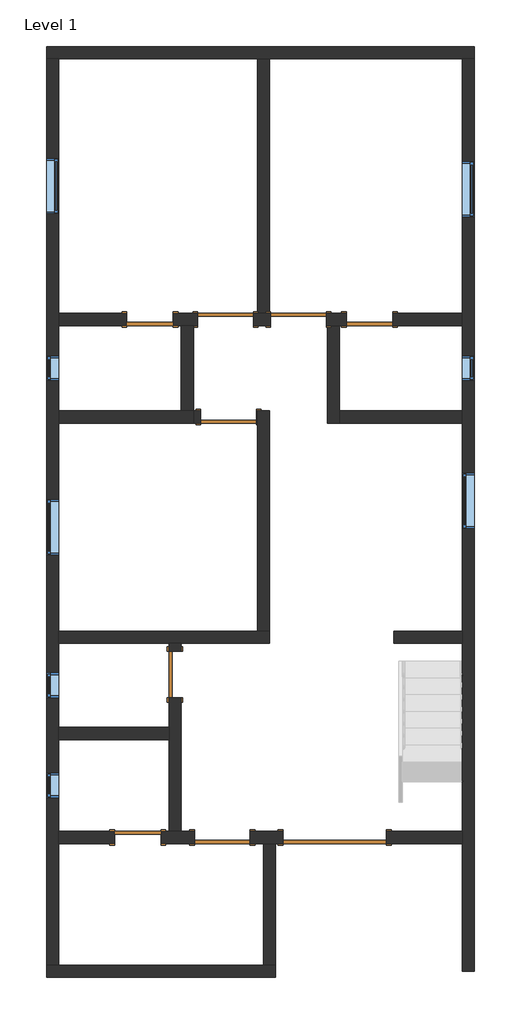
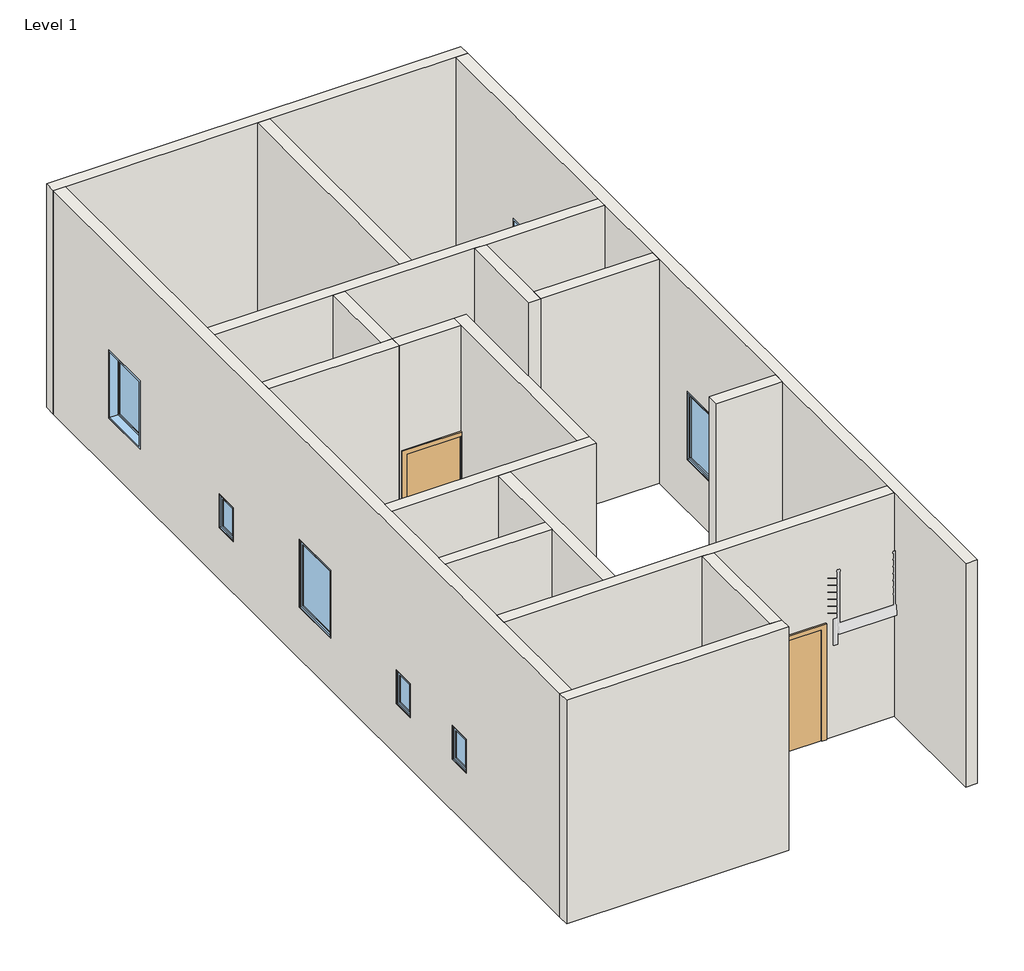
# One storey, part 1 of 2: 18 walls, 9 doors, 8 windows.
"""IFC4 building model written with IfcOpenShell, lengths in millimetres."""

from ifc_helpers import new_model, si_unit, frame, origin, origin_with_axes, place, context, project, spatial, polyline, outline, extrude, faceted_brep, transform, mapped, element, save
from components import m_door_double_flush_panel_double_acting_1700_x_2000mm_0a6d9c7f, m_single_flush_0762_x_2032mm_0c256fab, m_single_flush_0762_x_2032mm_7341a4fb, m_single_flush_0915_x_2032mm_26613924, m_single_flush_0915_x_2032mm_7267827e, m_single_flush_0915_x_2134mm_727434cd, m_fixed_0406_x_0610mm_8205b201, m_fixed_0915_x_1220mm_488fb2fb

model = new_model("IFC4")

# Units and contexts
model_context = context("Model", 3, world=origin())
ifc_project = project(units=[si_unit("LENGTHUNIT", "METRE", prefix="MILLI")], contexts=[model_context])

# Site, building, storey
site = spatial("IfcSite", under=ifc_project)
building = spatial("IfcBuilding", under=site)
storey = spatial("IfcBuildingStorey", under=building, Name="Level 1", Elevation=0.0)

# Doors
placement = place(None, origin())
m_door_double_flush_panel_double_acting_1700_x_2000mm_shape = m_door_double_flush_panel_double_acting_1700_x_2000mm_0a6d9c7f(model_context)
element("IfcDoor", 1, ObjectType="M_Door-Double-Flush_Panel-Double-Acting : 1700 x 2000mm", at=placement, inside=storey, context=model_context, shape_type="MappedRepresentation", body=[
    mapped(m_door_double_flush_panel_double_acting_1700_x_2000mm_shape, transform((-2797.9065777, -2525.6397347, 0.0), x_axis=(-1.0, 0.0, 0.0), y_axis=(0.0, -1.0, 0.0), z_axis=(0.0, 0.0, 1.0))),
])
m_single_flush_0762_x_2032mm_shape = m_single_flush_0762_x_2032mm_0c256fab(model_context)
element("IfcDoor", 2, ObjectType="M_Single-Flush : 0762 x 2032mm", at=placement, inside=storey, context=model_context, shape_type="MappedRepresentation", body=[
    mapped(m_single_flush_0762_x_2032mm_shape, transform((-6025.3065777, -2525.6397347, 0.0), x_axis=(1.0, 0.0, 0.0), y_axis=(0.0, 1.0, 0.0), z_axis=(0.0, 0.0, 1.0))),
])
element("IfcDoor", 3, ObjectType="M_Single-Flush : 0762 x 2032mm", at=placement, inside=storey, context=model_context, shape_type="MappedRepresentation", body=[
    mapped(m_single_flush_0762_x_2032mm_shape, transform((-5415.7065777, 141.3602653, 0.0), x_axis=(0.0, 1.0, 0.0), y_axis=(-1.0, 0.0, 0.0), z_axis=(0.0, 0.0, 1.0))),
])
element("IfcDoor", 4, ObjectType="M_Single-Flush : 0762 x 2032mm", at=placement, inside=storey, context=model_context, shape_type="MappedRepresentation", body=[
    mapped(m_single_flush_0762_x_2032mm_shape, transform((-2227.9565777, 5954.7602653, 0.0), x_axis=(-1.0, 0.0, 0.0), y_axis=(0.0, -1.0, 0.0), z_axis=(0.0, 0.0, 1.0))),
])
m_single_flush_0762_x_2032mm_2_shape = m_single_flush_0762_x_2032mm_7341a4fb(model_context)
element("IfcDoor", 5, ObjectType="M_Single-Flush : 0762 x 2032mm", at=placement, inside=storey, context=model_context, shape_type="MappedRepresentation", body=[
    mapped(m_single_flush_0762_x_2032mm_2_shape, transform((-5823.7065777, 5954.7602653, 0.0), x_axis=(1.0, 0.0, 0.0), y_axis=(0.0, 1.0, 0.0), z_axis=(0.0, 0.0, 1.0))),
])
m_single_flush_0915_x_2032mm_shape = m_single_flush_0915_x_2032mm_26613924(model_context)
element("IfcDoor", 6, ObjectType="M_Single-Flush : 0915 x 2032mm", at=placement, inside=storey, context=model_context, shape_type="MappedRepresentation", body=[
    mapped(m_single_flush_0915_x_2032mm_shape, transform((-4539.4065777, 4356.1602653, 0.0), x_axis=(1.0, 0.0, 0.0), y_axis=(0.0, 1.0, 0.0), z_axis=(0.0, 0.0, 1.0))),
])
element("IfcDoor", 7, ObjectType="M_Single-Flush : 0915 x 2032mm", at=placement, inside=storey, context=model_context, shape_type="MappedRepresentation", body=[
    mapped(m_single_flush_0915_x_2032mm_shape, transform((-3390.8065777, 5954.7602653, 0.0), x_axis=(-1.0, 0.0, 0.0), y_axis=(0.0, -1.0, 0.0), z_axis=(0.0, 0.0, 1.0))),
])
m_single_flush_0915_x_2032mm_2_shape = m_single_flush_0915_x_2032mm_7267827e(model_context)
element("IfcDoor", 8, ObjectType="M_Single-Flush : 0915 x 2032mm", at=placement, inside=storey, context=model_context, shape_type="MappedRepresentation", body=[
    mapped(m_single_flush_0915_x_2032mm_2_shape, transform((-4588.6065777, 5954.7602653, 0.0), x_axis=(1.0, 0.0, 0.0), y_axis=(0.0, 1.0, 0.0), z_axis=(0.0, 0.0, 1.0))),
])
m_single_flush_0915_x_2134mm_shape = m_single_flush_0915_x_2134mm_727434cd(model_context)
element("IfcDoor", 9, ObjectType="M_Single-Flush : 0915 x 2134mm", at=placement, inside=storey, context=model_context, shape_type="MappedRepresentation", body=[
    mapped(m_single_flush_0915_x_2134mm_shape, transform((-4640.2065777, -2525.6397347, 0.0), x_axis=(1.0, 0.0, 0.0), y_axis=(0.0, 1.0, 0.0), z_axis=(0.0, 0.0, 1.0))),
])

# Walls
element("IfcWall", 10, ObjectType="Generic - 200mm", at=placement, inside=storey, context=model_context, shape_type="Brep", body=[
    faceted_brep([(-7520.7065777, 10221.9602653, 0.0), (-7320.7065777, 10221.9602653, 0.0), (-4063.1065777, 10221.9602653, 0.0), (-3863.1065777, 10221.9602653, 0.0), (-710.3065777, 10221.9602653, 0.0), (-510.3065777, 10221.9602653, 0.0), (-510.3065777, 10221.9602653, 4000.0), (-710.3065777, 10221.9602653, 4000.0), (-3863.1065777, 10221.9602653, 4000.0), (-4063.1065777, 10221.9602653, 4000.0), (-7320.7065777, 10221.9602653, 4000.0), (-7520.7065777, 10221.9602653, 4000.0), (-7520.7065777, 10421.9602653, 0.0), (-7520.7065777, 10421.9602653, 4000.0), (-510.3065777, 10421.9602653, 4000.0), (-510.3065777, 10421.9602653, 0.0)], [[[0, 1, 2, 3, 4, 5, 6, 7, 8, 9, 10, 11]], [[12, 13, 14, 15]], [[5, 4, 3, 2, 1, 0, 12, 15]], [[11, 10, 9, 8, 7, 6, 14, 13]], [[6, 5, 15, 14]], [[0, 11, 13, 12]]]),
])
element("IfcWall", 11, ObjectType="Generic - 200mm", at=placement, inside=storey, context=model_context, shape_type="Brep", body=[
    faceted_brep([(-710.3065777, 10221.9602653, 0.0), (-710.3065777, 6054.7602653, 0.0), (-710.3065777, 5854.7602653, 0.0), (-710.3065777, 4456.1602653, 0.0), (-710.3065777, 4256.1602653, 0.0), (-710.3065777, 850.9602653, 0.0), (-710.3065777, 650.9602653, 0.0), (-710.3065777, -2425.6397347, 0.0), (-710.3065777, -2625.6397347, 0.0), (-710.3065777, -4718.0397347, 0.0), (-710.3065777, -4718.0397347, 4000.0), (-710.3065777, -2625.6397347, 4000.0), (-710.3065777, -2425.6397347, 4000.0), (-710.3065777, 650.9602653, 4000.0), (-710.3065777, 850.9602653, 4000.0), (-710.3065777, 4256.1602653, 4000.0), (-710.3065777, 4456.1602653, 4000.0), (-710.3065777, 5854.7602653, 4000.0), (-710.3065777, 6054.7602653, 4000.0), (-710.3065777, 10221.9602653, 4000.0), (-710.3065777, 5358.4602653, 915.0), (-710.3065777, 5358.4602653, 1525.0), (-710.3065777, 4952.4602653, 1525.0), (-710.3065777, 4952.4602653, 915.0), (-710.3065777, 8545.0602653, 915.0), (-710.3065777, 8545.0602653, 2135.0), (-710.3065777, 7630.0602653, 2135.0), (-710.3065777, 7630.0602653, 915.0), (-710.3065777, 2527.0602653, 2135.0), (-710.3065777, 2527.0602653, 915.0), (-710.3065777, 3442.0602653, 915.0), (-710.3065777, 3442.0602653, 2135.0), (-510.3065777, -4718.0397347, 0.0), (-510.3065777, 10221.9602653, 0.0), (-510.3065777, 10221.9602653, 4000.0), (-510.3065777, -4718.0397347, 4000.0), (-510.3065777, 5358.4602653, 1525.0), (-510.3065777, 5358.4602653, 915.0), (-510.3065777, 4952.4602653, 915.0), (-510.3065777, 4952.4602653, 1525.0), (-510.3065777, 8545.0602653, 2135.0), (-510.3065777, 8545.0602653, 915.0), (-510.3065777, 7630.0602653, 915.0), (-510.3065777, 7630.0602653, 2135.0), (-510.3065777, 2527.0602653, 915.0), (-510.3065777, 2527.0602653, 2135.0), (-510.3065777, 3442.0602653, 2135.0), (-510.3065777, 3442.0602653, 915.0)], [[[0, 1, 2, 3, 4, 5, 6, 7, 8, 9, 10, 11, 12, 13, 14, 15, 16, 17, 18, 19], [20, 21, 22, 23], [24, 25, 26, 27], [28, 29, 30, 31]], [[32, 33, 34, 35], [36, 37, 38, 39], [40, 41, 42, 43], [44, 45, 46, 47]], [[9, 8, 7, 6, 5, 4, 3, 2, 1, 0, 33, 32]], [[10, 9, 32, 35]], [[19, 18, 17, 16, 15, 14, 13, 12, 11, 10, 35, 34]], [[0, 19, 34, 33]], [[21, 20, 37, 36]], [[22, 21, 36, 39]], [[23, 22, 39, 38]], [[20, 23, 38, 37]], [[24, 41, 40, 25]], [[25, 40, 43, 26]], [[26, 43, 42, 27]], [[41, 24, 27, 42]], [[45, 44, 29, 28]], [[46, 45, 28, 31]], [[47, 46, 31, 30]], [[44, 47, 30, 29]]]),
])
element("IfcWall", 12, ObjectType="Generic - 200mm", at=placement, inside=storey, context=model_context, shape_type="Brep", body=[
    faceted_brep([(-3764.7065777, -4618.0397347, 0.0), (-3964.7065777, -4618.0397347, 0.0), (-7320.7065777, -4618.0397347, 0.0), (-7520.7065777, -4618.0397347, 0.0), (-7520.7065777, -4618.0397347, 4000.0), (-7320.7065777, -4618.0397347, 4000.0), (-3964.7065777, -4618.0397347, 4000.0), (-3764.7065777, -4618.0397347, 4000.0), (-3764.7065777, -4818.0397347, 0.0), (-3764.7065777, -4818.0397347, 4000.0), (-7520.7065777, -4818.0397347, 4000.0), (-7520.7065777, -4818.0397347, 0.0)], [[[0, 1, 2, 3, 4, 5, 6, 7]], [[8, 9, 10, 11]], [[3, 2, 1, 0, 8, 11]], [[7, 6, 5, 4, 10, 9]], [[4, 3, 11, 10]], [[0, 7, 9, 8]]]),
])
element("IfcWall", 13, ObjectType="Generic - 200mm", at=placement, inside=storey, context=model_context, shape_type="Brep", body=[
    faceted_brep([(-7320.7065777, -4618.0397347, 0.0), (-7320.7065777, -2625.6397347, 0.0), (-7320.7065777, -2425.6397347, 0.0), (-7320.7065777, -923.8397347, 0.0), (-7320.7065777, -723.8397347, 0.0), (-7320.7065777, 650.9602653, 0.0), (-7320.7065777, 850.9602653, 0.0), (-7320.7065777, 4256.1602653, 0.0), (-7320.7065777, 4456.1602653, 0.0), (-7320.7065777, 5854.7602653, 0.0), (-7320.7065777, 6054.7602653, 0.0), (-7320.7065777, 10221.9602653, 0.0), (-7320.7065777, 10221.9602653, 4000.0), (-7320.7065777, 6054.7602653, 4000.0), (-7320.7065777, 5854.7602653, 4000.0), (-7320.7065777, 4456.1602653, 4000.0), (-7320.7065777, 4256.1602653, 4000.0), (-7320.7065777, 850.9602653, 4000.0), (-7320.7065777, 650.9602653, 4000.0), (-7320.7065777, -723.8397347, 4000.0), (-7320.7065777, -923.8397347, 4000.0), (-7320.7065777, -2425.6397347, 4000.0), (-7320.7065777, -2625.6397347, 4000.0), (-7320.7065777, -4618.0397347, 4000.0), (-7320.7065777, 4952.4602653, 915.0), (-7320.7065777, 4952.4602653, 1525.0), (-7320.7065777, 5358.4602653, 1525.0), (-7320.7065777, 5358.4602653, 915.0), (-7320.7065777, -239.4397347, 915.0), (-7320.7065777, -239.4397347, 1525.0), (-7320.7065777, 166.5602653, 1525.0), (-7320.7065777, 166.5602653, 915.0), (-7320.7065777, -1877.7397347, 915.0), (-7320.7065777, -1877.7397347, 1525.0), (-7320.7065777, -1471.7397347, 1525.0), (-7320.7065777, -1471.7397347, 915.0), (-7320.7065777, 2096.0602653, 915.0), (-7320.7065777, 2096.0602653, 2135.0), (-7320.7065777, 3011.0602653, 2135.0), (-7320.7065777, 3011.0602653, 915.0), (-7320.7065777, 8595.8602653, 915.0), (-7320.7065777, 7680.8602653, 915.0), (-7320.7065777, 7680.8602653, 2135.0), (-7320.7065777, 8595.8602653, 2135.0), (-7520.7065777, -4618.0397347, 0.0), (-7520.7065777, -4618.0397347, 4000.0), (-7520.7065777, 10221.9602653, 4000.0), (-7520.7065777, 10221.9602653, 0.0), (-7520.7065777, 4952.4602653, 915.0), (-7520.7065777, 5358.4602653, 915.0), (-7520.7065777, 5358.4602653, 1525.0), (-7520.7065777, 4952.4602653, 1525.0), (-7520.7065777, -239.4397347, 915.0), (-7520.7065777, 166.5602653, 915.0), (-7520.7065777, 166.5602653, 1525.0), (-7520.7065777, -239.4397347, 1525.0), (-7520.7065777, -1877.7397347, 915.0), (-7520.7065777, -1471.7397347, 915.0), (-7520.7065777, -1471.7397347, 1525.0), (-7520.7065777, -1877.7397347, 1525.0), (-7520.7065777, 2096.0602653, 915.0), (-7520.7065777, 3011.0602653, 915.0), (-7520.7065777, 3011.0602653, 2135.0), (-7520.7065777, 2096.0602653, 2135.0), (-7520.7065777, 8595.8602653, 915.0), (-7520.7065777, 8595.8602653, 2135.0), (-7520.7065777, 7680.8602653, 2135.0), (-7520.7065777, 7680.8602653, 915.0)], [[[0, 1, 2, 3, 4, 5, 6, 7, 8, 9, 10, 11, 12, 13, 14, 15, 16, 17, 18, 19, 20, 21, 22, 23], [24, 25, 26, 27], [28, 29, 30, 31], [32, 33, 34, 35], [36, 37, 38, 39], [40, 41, 42, 43]], [[44, 45, 46, 47], [48, 49, 50, 51], [52, 53, 54, 55], [56, 57, 58, 59], [60, 61, 62, 63], [64, 65, 66, 67]], [[11, 10, 9, 8, 7, 6, 5, 4, 3, 2, 1, 0, 44, 47]], [[23, 22, 21, 20, 19, 18, 17, 16, 15, 14, 13, 12, 46, 45]], [[12, 11, 47, 46]], [[0, 23, 45, 44]], [[25, 24, 48, 51]], [[26, 25, 51, 50]], [[27, 26, 50, 49]], [[24, 27, 49, 48]], [[29, 28, 52, 55]], [[30, 29, 55, 54]], [[31, 30, 54, 53]], [[28, 31, 53, 52]], [[33, 32, 56, 59]], [[34, 33, 59, 58]], [[35, 34, 58, 57]], [[32, 35, 57, 56]], [[37, 36, 60, 63]], [[38, 37, 63, 62]], [[39, 38, 62, 61]], [[36, 39, 61, 60]], [[65, 64, 40, 43]], [[66, 65, 43, 42]], [[67, 66, 42, 41]], [[64, 67, 41, 40]]]),
])
element("IfcWall", 14, ObjectType="Generic - 200mm", at=placement, inside=storey, context=model_context, shape_type="Brep", body=[
    faceted_brep([(-5442.7065777, 5854.7602653, 2032.0), (-5442.7065777, 5854.7602653, 0.0), (-5314.1065777, 5854.7602653, 0.0), (-5114.1065777, 5854.7602653, 0.0), (-5046.1065777, 5854.7602653, 0.0), (-5046.1065777, 5854.7602653, 2032.0), (-4131.1065777, 5854.7602653, 2032.0), (-4131.1065777, 5854.7602653, 0.0), (-3848.3065777, 5854.7602653, 0.0), (-3848.3065777, 5854.7602653, 2032.0), (-2933.3065777, 5854.7602653, 2032.0), (-2933.3065777, 5854.7602653, 0.0), (-2918.5065777, 5854.7602653, 0.0), (-2718.5065777, 5854.7602653, 0.0), (-2608.9565777, 5854.7602653, 0.0), (-2608.9565777, 5854.7602653, 2032.0), (-1846.9565777, 5854.7602653, 2032.0), (-1846.9565777, 5854.7602653, 0.0), (-710.3065777, 5854.7602653, 0.0), (-710.3065777, 5854.7602653, 4000.0), (-2718.5065777, 5854.7602653, 4000.0), (-2918.5065777, 5854.7602653, 4000.0), (-5114.1065777, 5854.7602653, 4000.0), (-5314.1065777, 5854.7602653, 4000.0), (-7320.7065777, 5854.7602653, 4000.0), (-7320.7065777, 5854.7602653, 0.0), (-6204.7065777, 5854.7602653, 0.0), (-6204.7065777, 5854.7602653, 2032.0), (-5046.1065777, 6054.7602653, 0.0), (-5442.7065777, 6054.7602653, 0.0), (-5442.7065777, 6054.7602653, 2032.0), (-6204.7065777, 6054.7602653, 2032.0), (-6204.7065777, 6054.7602653, 0.0), (-7320.7065777, 6054.7602653, 0.0), (-7320.7065777, 6054.7602653, 4000.0), (-4063.1065777, 6054.7602653, 4000.0), (-3863.1065777, 6054.7602653, 4000.0), (-710.3065777, 6054.7602653, 4000.0), (-710.3065777, 6054.7602653, 0.0), (-1846.9565777, 6054.7602653, 0.0), (-1846.9565777, 6054.7602653, 2032.0), (-2608.9565777, 6054.7602653, 2032.0), (-2608.9565777, 6054.7602653, 0.0), (-2933.3065777, 6054.7602653, 0.0), (-2933.3065777, 6054.7602653, 2032.0), (-3848.3065777, 6054.7602653, 2032.0), (-3848.3065777, 6054.7602653, 0.0), (-3863.1065777, 6054.7602653, 0.0), (-4063.1065777, 6054.7602653, 0.0), (-4131.1065777, 6054.7602653, 0.0), (-4131.1065777, 6054.7602653, 2032.0), (-5046.1065777, 6054.7602653, 2032.0)], [[[0, 1, 2, 3, 4, 5, 6, 7, 8, 9, 10, 11, 12, 13, 14, 15, 16, 17, 18, 19, 20, 21, 22, 23, 24, 25, 26, 27]], [[28, 29, 30, 31, 32, 33, 34, 35, 36, 37, 38, 39, 40, 41, 42, 43, 44, 45, 46, 47, 48, 49, 50, 51]], [[8, 7, 49, 48, 47, 46]], [[39, 38, 18, 17]], [[43, 42, 14, 13, 12, 11]], [[26, 25, 33, 32]], [[4, 3, 2, 1, 29, 28]], [[24, 23, 22, 21, 20, 19, 37, 36, 35, 34]], [[19, 18, 38, 37]], [[25, 24, 34, 33]], [[9, 8, 46, 45]], [[10, 9, 45, 44]], [[11, 10, 44, 43]], [[50, 49, 7, 6]], [[51, 50, 6, 5]], [[28, 51, 5, 4]], [[15, 14, 42, 41]], [[16, 15, 41, 40]], [[17, 16, 40, 39]], [[30, 29, 1, 0]], [[31, 30, 0, 27]], [[32, 31, 27, 26]]]),
])
element("IfcWall", 15, ObjectType="Generic - 200mm", at=placement, inside=storey, context=model_context, shape_type="SweptSolid", body=[
    extrude(outline(polyline([(-4063.1065777, 6054.7602653), (-4063.1065777, 10221.9602653), (-3863.1065777, 10221.9602653), (-3863.1065777, 6054.7602653), (-4063.1065777, 6054.7602653)])), origin_with_axes(), (0.0, 0.0, 1.0), 4000.0),
])
element("IfcWall", 16, ObjectType="Generic - 200mm", at=placement, inside=storey, context=model_context, shape_type="Brep", body=[
    faceted_brep([(-7320.7065777, 4256.1602653, 0.0), (-5114.1065777, 4256.1602653, 0.0), (-5114.1065777, 4256.1602653, 4000.0), (-7320.7065777, 4256.1602653, 4000.0), (-7320.7065777, 4456.1602653, 0.0), (-7320.7065777, 4456.1602653, 4000.0), (-5314.1065777, 4456.1602653, 4000.0), (-5114.1065777, 4456.1602653, 4000.0), (-5114.1065777, 4456.1602653, 0.0), (-5314.1065777, 4456.1602653, 0.0)], [[[0, 1, 2, 3]], [[4, 5, 6, 7, 8, 9]], [[1, 0, 4, 9, 8]], [[3, 2, 7, 6, 5]], [[0, 3, 5, 4]], [[2, 1, 8, 7]]]),
])
element("IfcWall", 17, ObjectType="Generic - 200mm", at=placement, inside=storey, context=model_context, shape_type="SweptSolid", body=[
    extrude(outline(polyline([(-5114.1065777, 5854.7602653), (-5114.1065777, 4456.1602653), (-5314.1065777, 4456.1602653), (-5314.1065777, 5854.7602653), (-5114.1065777, 5854.7602653)])), origin_with_axes(), (0.0, 0.0, 1.0), 4000.0),
])
element("IfcWall", 18, ObjectType="Generic - 200mm", at=placement, inside=storey, context=model_context, shape_type="Brep", body=[
    faceted_brep([(-2918.5065777, 5854.7602653, 0.0), (-2918.5065777, 4256.1602653, 0.0), (-2918.5065777, 4256.1602653, 4000.0), (-2918.5065777, 5854.7602653, 4000.0), (-2718.5065777, 5854.7602653, 0.0), (-2718.5065777, 5854.7602653, 4000.0), (-2718.5065777, 4456.1602653, 4000.0), (-2718.5065777, 4256.1602653, 4000.0), (-2718.5065777, 4256.1602653, 0.0), (-2718.5065777, 4456.1602653, 0.0)], [[[0, 1, 2, 3]], [[4, 5, 6, 7, 8, 9]], [[1, 0, 4, 9, 8]], [[3, 2, 7, 6, 5]], [[0, 3, 5, 4]], [[2, 1, 8, 7]]]),
])
element("IfcWall", 19, ObjectType="Generic - 200mm", at=placement, inside=storey, context=model_context, shape_type="SweptSolid", body=[
    extrude(outline(polyline([(-710.3065777, 4256.1602653), (-2718.5065777, 4256.1602653), (-2718.5065777, 4456.1602653), (-710.3065777, 4456.1602653), (-710.3065777, 4256.1602653)])), origin_with_axes(), (0.0, 0.0, 1.0), 4000.0),
])
element("IfcWall", 20, ObjectType="Generic - 200mm", at=placement, inside=storey, context=model_context, shape_type="Brep", body=[
    faceted_brep([(-7320.7065777, 650.9602653, 0.0), (-5515.7065777, 650.9602653, 0.0), (-5315.7065777, 650.9602653, 0.0), (-3864.7065777, 650.9602653, 0.0), (-3864.7065777, 650.9602653, 4000.0), (-5315.7065777, 650.9602653, 4000.0), (-5515.7065777, 650.9602653, 4000.0), (-7320.7065777, 650.9602653, 4000.0), (-7320.7065777, 850.9602653, 0.0), (-7320.7065777, 850.9602653, 4000.0), (-4064.7065777, 850.9602653, 4000.0), (-3864.7065777, 850.9602653, 4000.0), (-3864.7065777, 850.9602653, 0.0), (-4064.7065777, 850.9602653, 0.0)], [[[0, 1, 2, 3, 4, 5, 6, 7]], [[8, 9, 10, 11, 12, 13]], [[3, 2, 1, 0, 8, 13, 12]], [[7, 6, 5, 4, 11, 10, 9]], [[0, 7, 9, 8]], [[4, 3, 12, 11]]]),
])
element("IfcWall", 21, ObjectType="Generic - 200mm", at=placement, inside=storey, context=model_context, shape_type="Brep", body=[
    faceted_brep([(-3864.7065777, 850.9602653, 0.0), (-3864.7065777, 4456.1602653, 0.0), (-3864.7065777, 4456.1602653, 4000.0), (-3864.7065777, 850.9602653, 4000.0), (-4064.7065777, 850.9602653, 0.0), (-4064.7065777, 850.9602653, 4000.0), (-4064.7065777, 4256.1602653, 4000.0), (-4064.7065777, 4456.1602653, 4000.0), (-4064.7065777, 4456.1602653, 0.0), (-4064.7065777, 4256.1602653, 0.0)], [[[0, 1, 2, 3]], [[4, 5, 6, 7, 8, 9]], [[1, 0, 4, 9, 8]], [[3, 2, 7, 6, 5]], [[0, 3, 5, 4]], [[2, 1, 8, 7]]]),
])
element("IfcWall", 22, ObjectType="Generic - 200mm", at=placement, inside=storey, context=model_context, shape_type="SweptSolid", body=[
    extrude(outline(polyline([(2032.0, -4081.9065777), (0.0, -4081.9065777), (0.0, -4064.7065777), (4000.0, -4064.7065777), (4000.0, -5114.1065777), (0.0, -5114.1065777), (0.0, -4996.9065777), (2032.0, -4996.9065777), (2032.0, -4081.9065777)])), frame((0.0, 4256.1602653, 0.0), z_axis=(0.0, 1.0, 0.0), x_axis=(0.0, 0.0, 1.0)), (0.0, 0.0, 1.0), 200.0),
])
element("IfcWall", 23, ObjectType="Generic - 200mm", at=placement, inside=storey, context=model_context, shape_type="SweptSolid", body=[
    extrude(outline(polyline([(-1829.5065777, 850.9602653), (-710.3065777, 850.9602653), (-710.3065777, 650.9602653), (-1829.5065777, 650.9602653), (-1829.5065777, 850.9602653)])), origin_with_axes(), (0.0, 0.0, 1.0), 4000.0),
])
element("IfcWall", 24, ObjectType="Generic - 200mm", at=placement, inside=storey, context=model_context, shape_type="SweptSolid", body=[
    extrude(outline(polyline([(-5515.7065777, -923.8397347), (-7320.7065777, -923.8397347), (-7320.7065777, -723.8397347), (-5515.7065777, -723.8397347), (-5515.7065777, -923.8397347)])), origin_with_axes(), (0.0, 0.0, 1.0), 4000.0),
])
element("IfcWall", 25, ObjectType="Generic - 200mm", at=placement, inside=storey, context=model_context, shape_type="Brep", body=[
    faceted_brep([(-5315.7065777, 522.3602653, 2032.0), (-5315.7065777, 522.3602653, 0.0), (-5315.7065777, 650.9602653, 0.0), (-5315.7065777, 650.9602653, 4000.0), (-5315.7065777, -2425.6397347, 4000.0), (-5315.7065777, -2425.6397347, 0.0), (-5315.7065777, -239.6397347, 0.0), (-5315.7065777, -239.6397347, 2032.0), (-5515.7065777, 650.9602653, 0.0), (-5515.7065777, 522.3602653, 0.0), (-5515.7065777, 522.3602653, 2032.0), (-5515.7065777, -239.6397347, 2032.0), (-5515.7065777, -239.6397347, 0.0), (-5515.7065777, -723.8397347, 0.0), (-5515.7065777, -923.8397347, 0.0), (-5515.7065777, -2425.6397347, 0.0), (-5515.7065777, -2425.6397347, 4000.0), (-5515.7065777, -923.8397347, 4000.0), (-5515.7065777, -723.8397347, 4000.0), (-5515.7065777, 650.9602653, 4000.0)], [[[0, 1, 2, 3, 4, 5, 6, 7]], [[8, 9, 10, 11, 12, 13, 14, 15, 16, 17, 18, 19]], [[6, 5, 15, 14, 13, 12]], [[2, 1, 9, 8]], [[4, 3, 19, 18, 17, 16]], [[3, 2, 8, 19]], [[5, 4, 16, 15]], [[10, 9, 1, 0]], [[11, 10, 0, 7]], [[12, 11, 7, 6]]]),
])
element("IfcWall", 26, ObjectType="Generic - 200mm", at=placement, inside=storey, context=model_context, shape_type="Brep", body=[
    faceted_brep([(-710.3065777, -2625.6397347, 4000.0), (-3764.7065777, -2625.6397347, 4000.0), (-3964.7065777, -2625.6397347, 4000.0), (-7320.7065777, -2625.6397347, 4000.0), (-7320.7065777, -2625.6397347, 0.0), (-6406.3065777, -2625.6397347, 0.0), (-6406.3065777, -2625.6397347, 2032.0), (-5644.3065777, -2625.6397347, 2032.0), (-5644.3065777, -2625.6397347, 0.0), (-5097.7065777, -2625.6397347, 0.0), (-5097.7065777, -2625.6397347, 2134.0), (-4182.7065777, -2625.6397347, 2134.0), (-4182.7065777, -2625.6397347, 0.0), (-3964.7065777, -2625.6397347, 0.0), (-3764.7065777, -2625.6397347, 0.0), (-3647.9065777, -2625.6397347, 0.0), (-3647.9065777, -2625.6397347, 2000.0), (-1947.9065777, -2625.6397347, 2000.0), (-1947.9065777, -2625.6397347, 0.0), (-710.3065777, -2625.6397347, 0.0), (-7320.7065777, -2425.6397347, 4000.0), (-5515.7065777, -2425.6397347, 4000.0), (-5315.7065777, -2425.6397347, 4000.0), (-710.3065777, -2425.6397347, 4000.0), (-710.3065777, -2425.6397347, 0.0), (-1947.9065777, -2425.6397347, 0.0), (-1947.9065777, -2425.6397347, 2000.0), (-3647.9065777, -2425.6397347, 2000.0), (-3647.9065777, -2425.6397347, 0.0), (-4182.7065777, -2425.6397347, 0.0), (-4182.7065777, -2425.6397347, 2134.0), (-5097.7065777, -2425.6397347, 2134.0), (-5097.7065777, -2425.6397347, 0.0), (-5315.7065777, -2425.6397347, 0.0), (-5515.7065777, -2425.6397347, 0.0), (-5644.3065777, -2425.6397347, 0.0), (-5644.3065777, -2425.6397347, 2032.0), (-6406.3065777, -2425.6397347, 2032.0), (-6406.3065777, -2425.6397347, 0.0), (-7320.7065777, -2425.6397347, 0.0)], [[[0, 1, 2, 3, 4, 5, 6, 7, 8, 9, 10, 11, 12, 13, 14, 15, 16, 17, 18, 19]], [[20, 21, 22, 23, 24, 25, 26, 27, 28, 29, 30, 31, 32, 33, 34, 35, 36, 37, 38, 39]], [[4, 39, 38, 5]], [[24, 19, 18, 25]], [[12, 29, 28, 15, 14, 13]], [[32, 9, 8, 35, 34, 33]], [[3, 2, 1, 0, 23, 22, 21, 20]], [[4, 3, 20, 39]], [[0, 19, 24, 23]], [[30, 29, 12, 11]], [[31, 30, 11, 10]], [[32, 31, 10, 9]], [[36, 35, 8, 7]], [[37, 36, 7, 6]], [[38, 37, 6, 5]], [[27, 16, 15, 28]], [[16, 27, 26, 17]], [[17, 26, 25, 18]]]),
])
element("IfcWall", 27, ObjectType="Generic - 200mm", at=placement, inside=storey, context=model_context, shape_type="SweptSolid", body=[
    extrude(outline(polyline([(-3964.7065777, -4618.0397347), (-3964.7065777, -2625.6397347), (-3764.7065777, -2625.6397347), (-3764.7065777, -4618.0397347), (-3964.7065777, -4618.0397347)])), origin_with_axes(), (0.0, 0.0, 1.0), 4000.0),
])

# Windows
m_fixed_0406_x_0610mm_shape = m_fixed_0406_x_0610mm_8205b201(model_context)
element("IfcWindow", 28, ObjectType="M_Fixed : 0406 x 0610mm", at=placement, inside=storey, context=model_context, shape_type="MappedRepresentation", body=[
    mapped(m_fixed_0406_x_0610mm_shape, transform((-7407.7065777, 5155.4602653, 0.0), x_axis=(0.0, 1.0, 0.0), y_axis=(-1.0, 0.0, 0.0), z_axis=(0.0, 0.0, 1.0))),
])
element("IfcWindow", 29, ObjectType="M_Fixed : 0406 x 0610mm", at=placement, inside=storey, context=model_context, shape_type="MappedRepresentation", body=[
    mapped(m_fixed_0406_x_0610mm_shape, transform((-623.3065777, 5155.4602653, 0.0), x_axis=(0.0, -1.0, 0.0), y_axis=(1.0, 0.0, 0.0), z_axis=(0.0, 0.0, 1.0))),
])
element("IfcWindow", 30, ObjectType="M_Fixed : 0406 x 0610mm", at=placement, inside=storey, context=model_context, shape_type="MappedRepresentation", body=[
    mapped(m_fixed_0406_x_0610mm_shape, transform((-7407.7065777, -36.4397347, 0.0), x_axis=(0.0, 1.0, 0.0), y_axis=(-1.0, 0.0, 0.0), z_axis=(0.0, 0.0, 1.0))),
])
element("IfcWindow", 31, ObjectType="M_Fixed : 0406 x 0610mm", at=placement, inside=storey, context=model_context, shape_type="MappedRepresentation", body=[
    mapped(m_fixed_0406_x_0610mm_shape, transform((-7407.7065777, -1674.7397347, 0.0), x_axis=(0.0, 1.0, 0.0), y_axis=(-1.0, 0.0, 0.0), z_axis=(0.0, 0.0, 1.0))),
])
m_fixed_0915_x_1220mm_shape = m_fixed_0915_x_1220mm_488fb2fb(model_context)
element("IfcWindow", 32, ObjectType="M_Fixed : 0915 x 1220mm", at=placement, inside=storey, context=model_context, shape_type="MappedRepresentation", body=[
    mapped(m_fixed_0915_x_1220mm_shape, transform((-7407.7065777, 2553.5602653, 0.0), x_axis=(0.0, 1.0, 0.0), y_axis=(-1.0, 0.0, 0.0), z_axis=(0.0, 0.0, 1.0))),
])
element("IfcWindow", 33, ObjectType="M_Fixed : 0915 x 1220mm", at=placement, inside=storey, context=model_context, shape_type="MappedRepresentation", body=[
    mapped(m_fixed_0915_x_1220mm_shape, transform((-7433.7065777, 8138.3602653, 0.0), x_axis=(0.0, -1.0, 0.0), y_axis=(1.0, 0.0, 0.0), z_axis=(0.0, 0.0, 1.0))),
])
element("IfcWindow", 34, ObjectType="M_Fixed : 0915 x 1220mm", at=placement, inside=storey, context=model_context, shape_type="MappedRepresentation", body=[
    mapped(m_fixed_0915_x_1220mm_shape, transform((-623.3065777, 8087.5602653, 0.0), x_axis=(0.0, -1.0, 0.0), y_axis=(1.0, 0.0, 0.0), z_axis=(0.0, 0.0, 1.0))),
])
element("IfcWindow", 35, ObjectType="M_Fixed : 0915 x 1220mm", at=placement, inside=storey, context=model_context, shape_type="MappedRepresentation", body=[
    mapped(m_fixed_0915_x_1220mm_shape, transform((-597.3065777, 2984.5602653, 0.0), x_axis=(0.0, 1.0, 0.0), y_axis=(-1.0, 0.0, 0.0), z_axis=(0.0, 0.0, 1.0))),
])

save(model, "model.ifc")

# Revit data of these elements
# Type "M_Door-Double-Flush_Panel-Double-Acting : 1700 x 2000mm"
#   Type Mark = "22"
#   Construction Type Id = "DOOR"
#   Assembly Code = "C1020"
#   Analytic Construction = "Wooden"
#   W = 850 mm
#   Thickness = 50 mm
#   Thermal Resistance (R) = 0.455703 (m²·K)/W
#   Swing Angle [instance default] = 90.00°
#   Heat Transfer Coefficient (U) = 2.19465 W/(m²·K)
#   Height = 2000 mm
#   Trim Projection Ext. = 25 mm
#   Trim Projection Int. = 25 mm
#   Trim Width Ext. = 80 mm
#   Trim Width Int. = 80 mm
#   Width = 1700 mm
#   Define Thermal Properties by = 1
#   Panel Material = Wood - Birch - Solid Stained Light Low Gloss
#   Trim Material = Paint - Sienna
#   Visual Light Transmittance = 0
#   Solar Heat Gain Coefficient = 0
#   Function = (empty or 0)
#   Wall Closure = (empty or 0)
# Type "M_Single-Flush : 0762 x 2032mm"
#   Type Mark = "19"
#   Thickness = 51 mm
#   Height = 2032 mm
#   Trim Projection Ext = 25 mm
#   Trim Projection Int = 25 mm
#   Trim Width = 76 mm
#   Width = 762 mm
#   Door Material = Door - Panel
#   Frame Material = Door - Frame
#   Function = (empty or 0)
#   Wall Closure = (empty or 0)
# Type "M_Single-Flush : 0915 x 2032mm"
#   Type Mark = "20"
#   Thickness = 51 mm
#   Height = 2032 mm
#   Trim Projection Ext = 25 mm
#   Trim Projection Int = 25 mm
#   Trim Width = 76 mm
#   Width = 915 mm
#   Door Material = Door - Panel
#   Frame Material = Door - Frame
#   Function = (empty or 0)
#   Wall Closure = (empty or 0)
# Type "M_Single-Flush : 0915 x 2134mm"
#   Type Mark = "15"
#   Thickness = 51 mm
#   Height = 2134 mm
#   Trim Projection Ext = 25 mm
#   Trim Projection Int = 25 mm
#   Trim Width = 76 mm
#   Width = 915 mm
#   Door Material = Door - Panel
#   Frame Material = Door - Frame
#   Function = (empty or 0)
#   Wall Closure = (empty or 0)
# Type "Generic - 200mm"
#   Layers, outside or top first: 200 mm no material (function 1)
# Type "M_Fixed : 0406 x 0610mm"
#   Type Mark = "10"
#   Height = 610 mm
#   Default Sill Height = 915 mm
#   Width = 406 mm
#   Window Inset = 19 mm
#   Frame Exterior Material = Sash
#   Frame Interior Material = Sash
#   Glass Pane Material = Glass
#   Sash = Sash
#   Wall Closure = (empty or 0)
# Type "M_Fixed : 0915 x 1220mm"
#   Type Mark = "15"
#   Height = 1220 mm
#   Default Sill Height = 915 mm
#   Width = 915 mm
#   Window Inset = 19 mm
#   Frame Exterior Material = Sash
#   Frame Interior Material = Sash
#   Glass Pane Material = Glass
#   Sash = Sash
#   Wall Closure = (empty or 0)
# Element 1 (IfcDoor, "M_Door-Double-Flush_Panel-Double-Acting : 1700 x 2000mm")
#   Swing Angle = 90.00°
#   Phase Created = New Construction
#   Materials on its faces: "Paint - Sienna", "Wood - Birch - Solid Stained Light Low Gloss"
# Elements 2, 3, 4, 5 (IfcDoor, "M_Single-Flush : 0762 x 2032mm")
#   Phase Created = New Construction
#   Materials on its faces: "Door - Frame", "Door - Panel"
# Elements 6, 7, 8 (IfcDoor, "M_Single-Flush : 0915 x 2032mm")
#   Phase Created = New Construction
#   Materials on its faces: "Door - Frame", "Door - Panel"
# Element 9 (IfcDoor, "M_Single-Flush : 0915 x 2134mm")
#   Phase Created = New Construction
#   Materials on its faces: "Door - Frame", "Door - Panel"
# Elements 10, 11, 12, 13, 14, 15, 16, 17, 18, 19, 20, 21, 22, 23, 24, 25, 26, 27 (IfcWall, "Generic - 200mm")
#   Top Offset = 0 mm
#   Base Offset = 0 mm
#   wall height = 4000 mm
#   Phase Created = New Construction
#   Base Constraint = Level 1
#   Top Constraint = Level 2
#   Materials on its faces: "Default Wall"
# Element 28 (IfcWindow, "M_Fixed : 0406 x 0610mm")
#   Mark = "7"
#   Phase Created = New Construction
#   Materials on its faces: "Sash", "Glass"
# Element 29 (IfcWindow, "M_Fixed : 0406 x 0610mm")
#   Mark = "8"
#   Phase Created = New Construction
#   Materials on its faces: "Sash", "Glass"
# Element 30 (IfcWindow, "M_Fixed : 0406 x 0610mm")
#   Mark = "9"
#   Phase Created = New Construction
#   Materials on its faces: "Sash", "Glass"
# Element 31 (IfcWindow, "M_Fixed : 0406 x 0610mm")
#   Mark = "10"
#   Phase Created = New Construction
#   Materials on its faces: "Sash", "Glass"
# Element 32 (IfcWindow, "M_Fixed : 0915 x 1220mm")
#   Mark = "11"
#   Phase Created = New Construction
#   Materials on its faces: "Sash", "Glass"
# Element 33 (IfcWindow, "M_Fixed : 0915 x 1220mm")
#   Mark = "12"
#   Phase Created = New Construction
#   Materials on its faces: "Sash", "Glass"
# Element 34 (IfcWindow, "M_Fixed : 0915 x 1220mm")
#   Mark = "13"
#   Phase Created = New Construction
#   Materials on its faces: "Sash", "Glass"
# Element 35 (IfcWindow, "M_Fixed : 0915 x 1220mm")
#   Mark = "14"
#   Phase Created = New Construction
#   Materials on its faces: "Sash", "Glass"
# Materials
#   "Wood - Birch - Solid Stained Light Low Gloss": class "Wood", colour RGB 210 159 95, transparency 0, Cost = 0
#   "Paint - Sienna": colour RGB 118 70 51, transparency 0, Cost = 0
#   "Door - Panel": class "Wood", colour RGB 114 82 51, transparency 0
#   "Door - Frame": colour RGB 153 76 43, transparency 0
#   "Sash": class "Wood", colour RGB 136 99 55, transparency 0
#   "Glass": class "Glass", colour RGB 218 227 224, transparency 0.85, Description = "Soda Lime Glass", Cost = 0
#   "Default Wall": colour RGB 80 80 80, transparency 0
